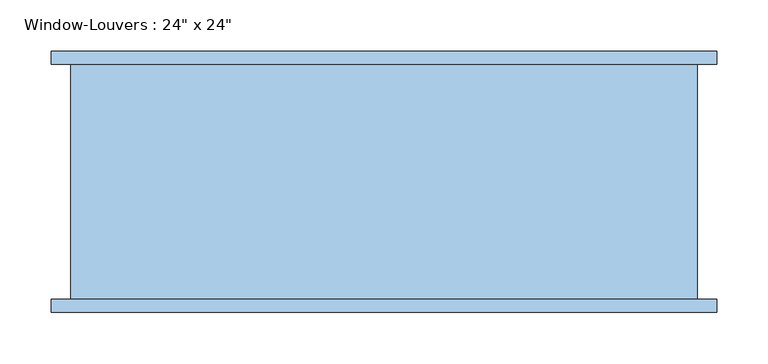
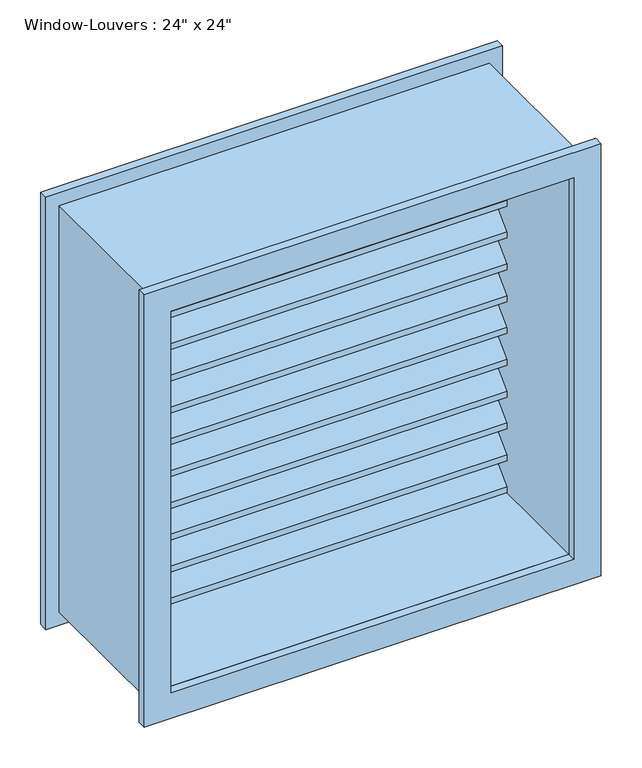
"""IFC4 building model written with IfcOpenShell, lengths in millimetres: window geometry."""

from ifc_helpers import new_model, si_unit, frame, origin, place, context, project, spatial, polyline, outline, extrude, source, transform, mapped, element, save


def window_f2d8fef0(model_context):
    return source(origin(), model_context, "Body", "SweptSolid", [
        extrude(outline(polyline([(107.95, 1419.1754778), (107.95, 1410.1952217), (69.85, 1448.2952217), (31.75, 1410.1952217), (31.75, 1419.1754778), (69.85, 1457.2754778), (107.95, 1419.1754778)])), frame((-285.75, 0.0, 0.0), z_axis=(1.0, 0.0, 0.0), x_axis=(0.0, 1.0, 0.0)), (0.0, 0.0, 1.0), 571.5),
        extrude(outline(polyline([(107.95, 1371.5009557), (107.95, 1362.5206995), (69.85, 1400.6206995), (31.75, 1362.5206995), (31.75, 1371.5009557), (69.85, 1409.6009557), (107.95, 1371.5009557)])), frame((-285.75, 0.0, 0.0), z_axis=(1.0, 0.0, 0.0), x_axis=(0.0, 1.0, 0.0)), (0.0, 0.0, 1.0), 571.5),
        extrude(outline(polyline([(107.95, 1323.8264335), (107.95, 1314.8461774), (69.85, 1352.9461774), (31.75, 1314.8461774), (31.75, 1323.8264335), (69.85, 1361.9264335), (107.95, 1323.8264335)])), frame((-285.75, 0.0, 0.0), z_axis=(1.0, 0.0, 0.0), x_axis=(0.0, 1.0, 0.0)), (0.0, 0.0, 1.0), 571.5),
        extrude(outline(polyline([(107.95, 1276.1519113), (107.95, 1267.1716552), (69.85, 1305.2716552), (31.75, 1267.1716552), (31.75, 1276.1519113), (69.85, 1314.2519113), (107.95, 1276.1519113)])), frame((-285.75, 0.0, 0.0), z_axis=(1.0, 0.0, 0.0), x_axis=(0.0, 1.0, 0.0)), (0.0, 0.0, 1.0), 571.5),
        extrude(outline(polyline([(107.95, 1228.4773891), (107.95, 1219.497133), (69.85, 1257.597133), (31.75, 1219.497133), (31.75, 1228.4773891), (69.85, 1266.5773891), (107.95, 1228.4773891)])), frame((-285.75, 0.0, 0.0), z_axis=(1.0, 0.0, 0.0), x_axis=(0.0, 1.0, 0.0)), (0.0, 0.0, 1.0), 571.5),
        extrude(outline(polyline([(107.95, 1180.802867), (107.95, 1171.8226109), (69.85, 1209.9226109), (31.75, 1171.8226109), (31.75, 1180.802867), (69.85, 1218.902867), (107.95, 1180.802867)])), frame((-285.75, 0.0, 0.0), z_axis=(1.0, 0.0, 0.0), x_axis=(0.0, 1.0, 0.0)), (0.0, 0.0, 1.0), 571.5),
        extrude(outline(polyline([(107.95, 1133.1283448), (107.95, 1124.1480887), (69.85, 1162.2480887), (31.75, 1124.1480887), (31.75, 1133.1283448), (69.85, 1171.2283448), (107.95, 1133.1283448)])), frame((-285.75, 0.0, 0.0), z_axis=(1.0, 0.0, 0.0), x_axis=(0.0, 1.0, 0.0)), (0.0, 0.0, 1.0), 571.5),
        extrude(outline(polyline([(107.95, 1085.4538226), (107.95, 1076.4735665), (69.85, 1114.5735665), (31.75, 1076.4735665), (31.75, 1085.4538226), (69.85, 1123.5538226), (107.95, 1085.4538226)])), frame((-285.75, 0.0, 0.0), z_axis=(1.0, 0.0, 0.0), x_axis=(0.0, 1.0, 0.0)), (0.0, 0.0, 1.0), 571.5),
        extrude(outline(polyline([(107.95, 1037.7793005), (107.95, 1028.7990443), (69.85, 1066.8990443), (31.75, 1028.7990443), (31.75, 1037.7793005), (69.85, 1075.8793005), (107.95, 1037.7793005)])), frame((-285.75, 0.0, 0.0), z_axis=(1.0, 0.0, 0.0), x_axis=(0.0, 1.0, 0.0)), (0.0, 0.0, 1.0), 571.5),
        extrude(outline(polyline([(107.95, 990.1047783), (107.95, 981.1245222), (69.85, 1019.2245222), (31.75, 981.1245222), (31.75, 990.1047783), (69.85, 1028.2047783), (107.95, 990.1047783)])), frame((-285.75, 0.0, 0.0), z_axis=(1.0, 0.0, 0.0), x_axis=(0.0, 1.0, 0.0)), (0.0, 0.0, 1.0), 571.5),
        extrude(outline(polyline([(107.95, 1466.85), (107.95, 1457.8697439), (69.85, 1495.9697439), (31.75, 1457.8697439), (31.75, 1466.85), (69.85, 1504.95), (107.95, 1466.85)])), frame((-285.75, 0.0, 0.0), z_axis=(1.0, 0.0, 0.0), x_axis=(0.0, 1.0, 0.0)), (0.0, 0.0, 1.0), 571.5),
        extrude(outline(polyline([(107.95, 942.4302561), (107.95, 933.45), (69.85, 971.55), (31.75, 933.45), (31.75, 942.4302561), (69.85, 980.5302561), (107.95, 942.4302561)])), frame((-285.75, 0.0, 0.0), z_axis=(1.0, 0.0, 0.0), x_axis=(0.0, 1.0, 0.0)), (0.0, 0.0, 1.0), 571.5),
        extrude(outline(polyline([(1524.0, 304.8), (1524.0, -304.8), (914.4, -304.8), (914.4, 304.8), (1524.0, 304.8)]), holes=[polyline([(1504.95, 285.75), (933.45, 285.75), (933.45, -285.75), (1504.95, -285.75), (1504.95, 285.75)])]), frame((0.0, -120.65, 0.0), z_axis=(0.0, 1.0, 0.0), x_axis=(0.0, 0.0, 1.0)), (0.0, 0.0, 1.0), 228.6),
        extrude(outline(polyline([(1543.05, 323.85), (1543.05, -323.85), (895.35, -323.85), (895.35, 323.85), (1543.05, 323.85)]), holes=[polyline([(1504.95, 285.75), (933.45, 285.75), (933.45, -285.75), (1504.95, -285.75), (1504.95, 285.75)])]), frame((0.0, -133.35, 0.0), z_axis=(0.0, 1.0, 0.0), x_axis=(0.0, 0.0, 1.0)), (0.0, 0.0, 1.0), 12.7),
        extrude(outline(polyline([(1543.05, -323.85), (895.35, -323.85), (895.35, 323.85), (1543.05, 323.85), (1543.05, -323.85)]), holes=[polyline([(1504.95, -285.75), (1504.95, 285.75), (933.45, 285.75), (933.45, -285.75), (1504.95, -285.75)])]), frame((0.0, 107.95, 0.0), z_axis=(0.0, 1.0, 0.0), x_axis=(0.0, 0.0, 1.0)), (0.0, 0.0, 1.0), 12.7),
    ])


if __name__ == "__main__":
    model = new_model("IFC4")
    model_context = context("Model", 3, world=origin())
    ifc_project = project(units=[si_unit("LENGTHUNIT", "METRE", prefix="MILLI")], contexts=[model_context])
    site = spatial("IfcSite", under=ifc_project)
    building = spatial("IfcBuilding", under=site)
    placement = place(None, origin())
    window_shape = window_f2d8fef0(model_context)
    element("IfcWindow", 1, ObjectType="Window-Louvers : 24\" x 24\"", at=placement, inside=building, context=model_context, shape_type="MappedRepresentation", body=[
        mapped(window_shape, transform((0.0, 0.0, 0.0), x_axis=(1.0, 0.0, 0.0), y_axis=(0.0, 1.0, 0.0), z_axis=(0.0, 0.0, 1.0))),
    ])
    save(model, "model.ifc")

# Revit data of these elements
# Type "Window-Louvers : 24\" x 24\""
#   Type Mark = "26"
#   Construction Type Id = "GSP4R"
#   Assembly Code = "B20"
#   Analytic Construction = "1/8 in Pilkington single glazing"
#   Visual Light Transmittance = 0.9
#   Thermal Resistance (R) = 1.53941 (h·ft²·°F)/BTU
#   Solar Heat Gain Coefficient = 0.78
#   Max Height = 1.978553 ft
#   Height = 2 ft
#   Heat Transfer Coefficient (U) = 0.6496 BTU/(h·ft²·°F)
#   Blade Width [instance default] = 1.875 ft
#   Blade Vertical Thickness = 0.029463 ft
#   Blade Thickness = 0.020833 ft
#   Blade Spacing = 0.125 ft
#   Blade Height = 0.154463 ft
#   Blade Depth = 0.25 ft
#   Blade Angle = 45.00°
#   Default Sill Height = 3 ft
#   Trim Projection_Exterior = 0.041667 ft
#   Trim Projection_Interior = 0.041667 ft
#   Trim Width_Exterior = 0.125 ft
#   Trim Width_Interior = 0.125 ft
#   Width = 2 ft
#   Max Blade Count = 12
#   Define Thermal Properties by = 1
#   Blade Count = 12
#   Frame Material = Birch
#   Louver Material = Birch
#   Trim Exterior Material = Birch
#   Trim Interior Material = Birch
#   Wall Closure = (empty or 0)
# Element 1 (IfcWindow, "Window-Louvers : 24\" x 24\"")
#   Materials on its faces: "Birch"
# Materials
#   "Birch": class "Wood", colour RGB 224 178 126, transparency 0, Description = "Betula Alleghaniensis", Cost = 0
